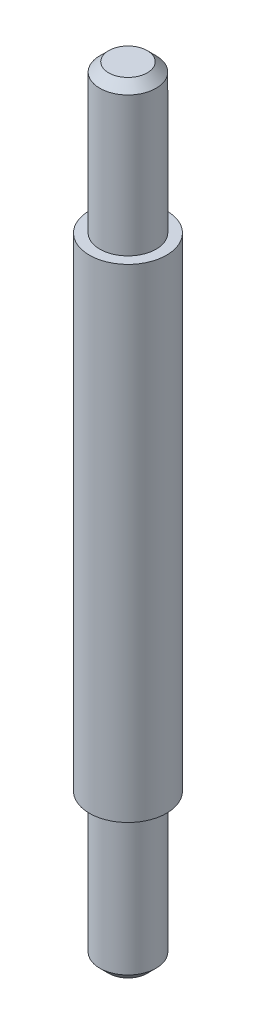
SolidWorks part; units mm, degrees
material "Plain Carbon Steel"
ref_plane "Front Plane" through (0, 0, 0) normal (0, 0, 1) x (1, 0, 0)
ref_plane "Top Plane" through (0, 0, 0) normal (0, 1, 0) x (1, 0, 0)
ref_plane "Right Plane" through (0, 0, 0) normal (1, 0, 0) x (0, 0, -1)
sketch "Pin Profile Sketch" plane through (0, 0, 0) normal (0, 0, 1) x (1, 0, 0)
  line L0 (0, 65.5594) -> (0, -68.005) construction
  line L1 (0, 131.5) -> (9.5, 131.5)
  line L2 (9.5, 131.5) -> (9.5, 81.5)
  line L3 (9.5, 81.5) -> (13, 81.5)
  line L4 (13, 81.5) -> (13, -81.5)
  line L5 (13, -81.5) -> (9.5, -81.5)
  line L6 (9.5, -81.5) -> (9.5, -131.5)
  line L7 (9.5, -131.5) -> (0, -131.5)
  line L8 (0, -131.5) -> (0, 131.5)
  dimension "D1" = 9.5
  dimension "D2" = 13
  dimension "D3" = 263
  dimension "D4" = 163
  dimension "D5" = 81.5
  dimension "D6" = 131.5
revolve "Pin Body Revolve" add sketch "Pin Profile Sketch" angle 360 about L0
chamfer "End Chamfers 3x45°" distance 3 angle 45 2 edges at (0, -131.5, 9.5) (0, 131.5, 9.5)
